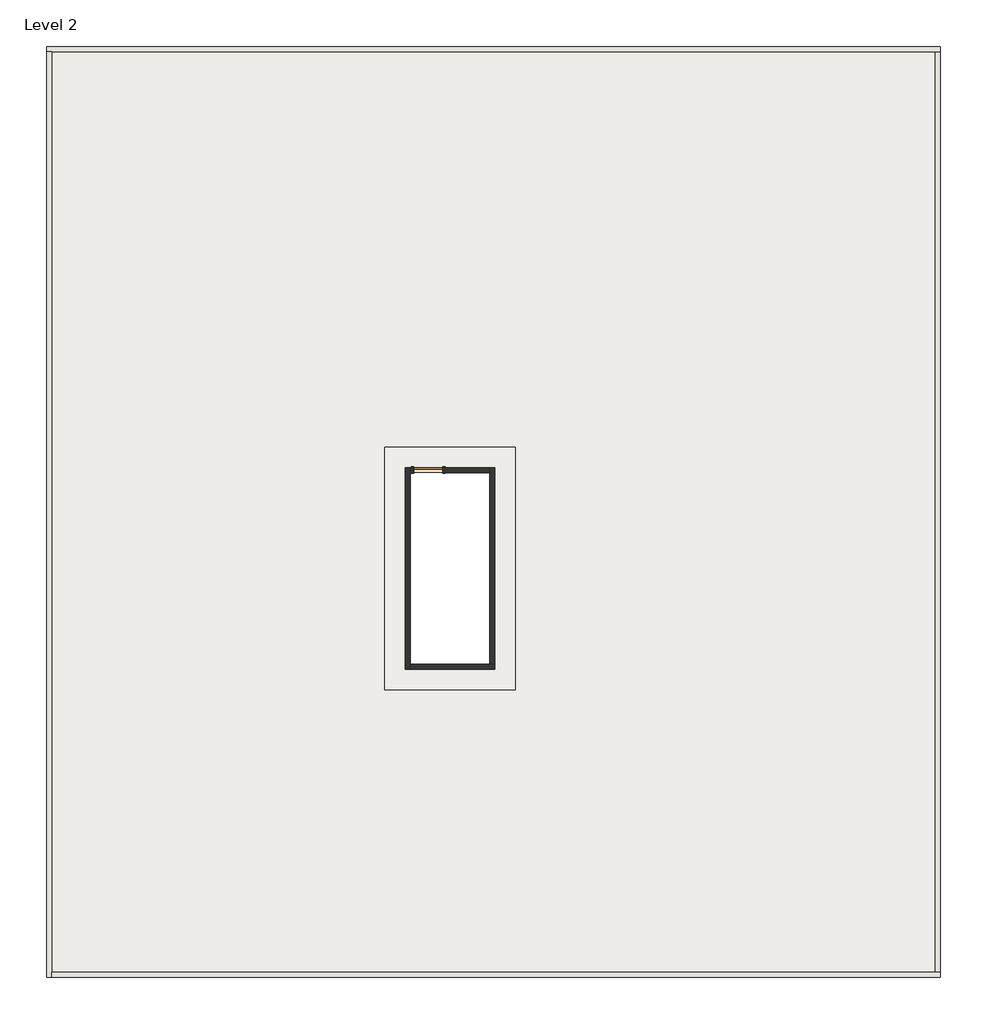
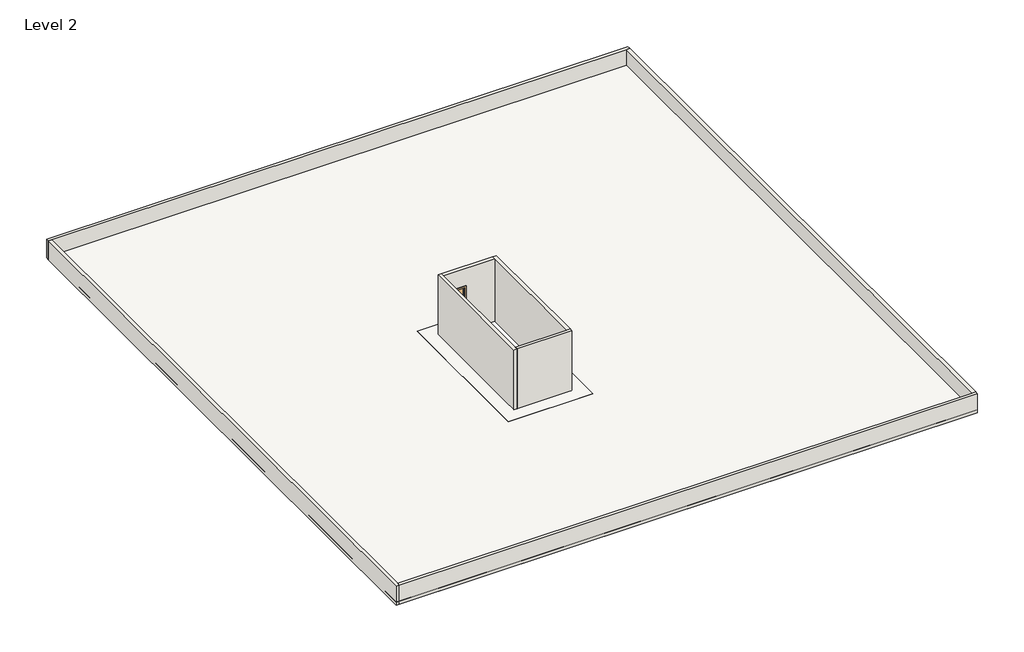
# One storey: 8 walls, 2 roofs, 1 door.
"""IFC4 building model written with IfcOpenShell, lengths in millimetres."""

from ifc_helpers import new_model, si_unit, frame, origin, place, context, project, spatial, polyline, outline, extrude, faceted_brep, transform, mapped, element, save
from components import door_b6e9fca3

model = new_model("IFC4")

# Units and contexts
model_context = context("Model", 3, world=origin())
ifc_project = project(units=[si_unit("LENGTHUNIT", "METRE", prefix="MILLI")], contexts=[model_context])

# Site, building, storey
site = spatial("IfcSite", under=ifc_project)
building = spatial("IfcBuilding", under=site)
storey = spatial("IfcBuildingStorey", under=building, Name="Level 2", Elevation=3048.0)

# Door
placement = place(None, origin())
door_shape = door_b6e9fca3(model_context)
element("IfcDoor", 1, ObjectType="Single-Flush : 34\" x 84\"", at=placement, inside=storey, context=model_context, shape_type="MappedRepresentation", body=[
    mapped(door_shape, transform((-2969.7844485, 1789.3269271, 3048.0), x_axis=(1.0, 0.0, 0.0), y_axis=(0.0, 1.0, 0.0), z_axis=(0.0, 0.0, 1.0))),
])

# Roofs
element("IfcRoof", 2, ObjectType="SLAB", at=placement, inside=storey, context=model_context, shape_type="SweptSolid", body=[
    extrude(outline(polyline([(12308.4014317, 14431.9935985), (12308.4014317, -13355.6064015), (-14366.7474256, -13355.6064015), (-14366.7474256, 14431.9935985), (12308.4014317, 14431.9935985)]), holes=[polyline([(-3503.1844485, 1713.1269271), (-3503.1844485, -4001.8730729), (-1140.9844485, -4001.8730729), (-1140.9844485, 1713.1269271), (-3503.1844485, 1713.1269271)])]), frame((0.0, 0.0, 3048.0), z_axis=(0.0, 0.0, 1.0), x_axis=(1.0, 0.0, 0.0)), (0.0, 0.0, 1.0), 152.4),
])
element("IfcRoof", 3, ObjectType="SLAB", at=placement, inside=storey, context=model_context, shape_type="SweptSolid", body=[
    extrude(outline(polyline([(-378.9844485, -4763.8730729), (-4265.1844485, -4763.8730729), (-4265.1844485, 2475.1269271), (-378.9844485, 2475.1269271), (-378.9844485, -4763.8730729)]), holes=[polyline([(-3503.1844485, 1713.1269271), (-3503.1844485, -4001.8730729), (-1140.9844485, -4001.8730729), (-1140.9844485, 1713.1269271), (-3503.1844485, 1713.1269271)])]), frame((0.0, 0.0, 3048.0), z_axis=(0.0, 0.0, 1.0), x_axis=(1.0, 0.0, 0.0)), (0.0, 0.0, 1.0), 152.4),
])

# Walls
element("IfcWall", 4, ObjectType="6\"", at=placement, inside=storey, context=model_context, shape_type="Brep", body=[
    faceted_brep([(-3655.5844485, 1865.5269271, 3048.0), (-3655.5844485, -4154.2730729, 3048.0), (-3655.5844485, -4154.2730729, 6096.0), (-3655.5844485, 1865.5269271, 6096.0), (-3503.1844485, 1865.5269271, 3048.0), (-3503.1844485, 1865.5269271, 6096.0), (-3503.1844485, 1713.1269271, 6096.0), (-3503.1844485, -4001.8730729, 6096.0), (-3503.1844485, -4154.2730729, 6096.0), (-3503.1844485, -4154.2730729, 3048.0), (-3503.1844485, -4001.8730729, 3048.0), (-3503.1844485, 1713.1269271, 3048.0)], [[[0, 1, 2, 3]], [[4, 5, 6, 7, 8, 9, 10, 11]], [[1, 0, 4, 11, 10, 9]], [[2, 1, 9, 8]], [[0, 3, 5, 4]], [[3, 2, 8, 7, 6, 5]]]),
])
element("IfcWall", 5, ObjectType="6\"", at=placement, inside=storey, context=model_context, shape_type="Brep", body=[
    faceted_brep([(-3503.1844485, -4154.2730729, 3048.0), (-988.5844485, -4154.2730729, 3048.0), (-988.5844485, -4154.2730729, 6096.0), (-3503.1844485, -4154.2730729, 6096.0), (-3503.1844485, -4001.8730729, 3048.0), (-3503.1844485, -4001.8730729, 6096.0), (-1140.9844485, -4001.8730729, 6096.0), (-988.5844485, -4001.8730729, 6096.0), (-988.5844485, -4001.8730729, 3048.0), (-1140.9844485, -4001.8730729, 3048.0)], [[[0, 1, 2, 3]], [[4, 5, 6, 7, 8, 9]], [[1, 0, 4, 9, 8]], [[0, 3, 5, 4]], [[2, 1, 8, 7]], [[3, 2, 7, 6, 5]]]),
])
element("IfcWall", 6, ObjectType="6\"", at=placement, inside=storey, context=model_context, shape_type="Brep", body=[
    faceted_brep([(-988.5844485, -4001.8730729, 3048.0), (-988.5844485, 1865.5269271, 3048.0), (-988.5844485, 1865.5269271, 6096.0), (-988.5844485, -4001.8730729, 6096.0), (-1140.9844485, -4001.8730729, 3048.0), (-1140.9844485, -4001.8730729, 6096.0), (-1140.9844485, 1713.1269271, 6096.0), (-1140.9844485, 1865.5269271, 6096.0), (-1140.9844485, 1865.5269271, 3048.0), (-1140.9844485, 1713.1269271, 3048.0)], [[[0, 1, 2, 3]], [[4, 5, 6, 7, 8, 9]], [[1, 0, 4, 9, 8]], [[0, 3, 5, 4]], [[2, 1, 8, 7]], [[3, 2, 7, 6, 5]]]),
])
element("IfcWall", 7, ObjectType="6\"", at=placement, inside=storey, context=model_context, shape_type="SweptSolid", body=[
    extrude(outline(polyline([(5181.6, -2537.9844485), (3048.0, -2537.9844485), (3048.0, -1140.9844485), (6096.0, -1140.9844485), (6096.0, -3503.1844485), (3048.0, -3503.1844485), (3048.0, -3401.5844485), (5181.6, -3401.5844485), (5181.6, -2537.9844485)])), frame((0.0, 1713.1269271, 0.0), z_axis=(0.0, 1.0, 0.0), x_axis=(0.0, 0.0, 1.0)), (0.0, 0.0, 1.0), 152.4),
])
element("IfcWall", 8, ObjectType="6\" 2", at=placement, inside=storey, context=model_context, shape_type="Brep", body=[
    faceted_brep([(12308.4014317, 14431.9935985, 3048.0), (-14366.7474256, 14431.9935985, 3048.0), (-14366.7474256, 14431.9935985, 3962.4), (12308.4014317, 14431.9935985, 3962.4), (12308.4014317, 14279.5935985, 3048.0), (12308.4014317, 14279.5935985, 3962.4), (12156.0014317, 14279.5935985, 3962.4), (-14214.3474256, 14279.5935985, 3962.4), (-14366.7474256, 14279.5935985, 3962.4), (-14366.7474256, 14279.5935985, 3048.0), (-14214.3474256, 14279.5935985, 3048.0), (12156.0014317, 14279.5935985, 3048.0)], [[[0, 1, 2, 3]], [[4, 5, 6, 7, 8, 9, 10, 11]], [[1, 0, 4, 11, 10, 9]], [[3, 2, 8, 7, 6, 5]], [[2, 1, 9, 8]], [[0, 3, 5, 4]]]),
])
element("IfcWall", 9, ObjectType="6\" 2", at=placement, inside=storey, context=model_context, shape_type="Brep", body=[
    faceted_brep([(-14366.7474256, 14279.5935985, 3048.0), (-14366.7474256, -13355.6064015, 3048.0), (-14366.7474256, -13355.6064015, 3962.4), (-14366.7474256, 14279.5935985, 3962.4), (-14214.3474256, 14279.5935985, 3048.0), (-14214.3474256, 14279.5935985, 3962.4), (-14214.3474256, -13203.2064015, 3962.4), (-14214.3474256, -13355.6064015, 3962.4), (-14214.3474256, -13355.6064015, 3048.0), (-14214.3474256, -13203.2064015, 3048.0)], [[[0, 1, 2, 3]], [[4, 5, 6, 7, 8, 9]], [[1, 0, 4, 9, 8]], [[3, 2, 7, 6, 5]], [[0, 3, 5, 4]], [[2, 1, 8, 7]]]),
])
element("IfcWall", 10, ObjectType="6\" 2", at=placement, inside=storey, context=model_context, shape_type="Brep", body=[
    faceted_brep([(-14214.3474256, -13355.6064015, 3048.0), (12308.4014317, -13355.6064015, 3048.0), (12308.4014317, -13355.6064015, 3962.4), (-14214.3474256, -13355.6064015, 3962.4), (-14214.3474256, -13203.2064015, 3048.0), (-14214.3474256, -13203.2064015, 3962.4), (12156.0014317, -13203.2064015, 3962.4), (12308.4014317, -13203.2064015, 3962.4), (12308.4014317, -13203.2064015, 3048.0), (12156.0014317, -13203.2064015, 3048.0)], [[[0, 1, 2, 3]], [[4, 5, 6, 7, 8, 9]], [[1, 0, 4, 9, 8]], [[3, 2, 7, 6, 5]], [[0, 3, 5, 4]], [[2, 1, 8, 7]]]),
])
element("IfcWall", 11, ObjectType="6\" 2", at=placement, inside=storey, context=model_context, shape_type="SweptSolid", body=[
    extrude(outline(polyline([(12308.4014317, 14279.5935985), (12308.4014317, -13203.2064015), (12156.0014317, -13203.2064015), (12156.0014317, 14279.5935985), (12308.4014317, 14279.5935985)])), frame((0.0, 0.0, 3048.0), z_axis=(0.0, 0.0, 1.0), x_axis=(1.0, 0.0, 0.0)), (0.0, 0.0, 1.0), 914.4),
])

save(model, "model.ifc")

# Revit data of these elements
# Type "Single-Flush : 34\" x 84\""
#   Type Mark = "2"
#   Construction Type Id = "MDOOR"
#   Assembly Code = "C1020"
#   Analytic Construction = "Metal"
#   Thickness = 0' - 2"
#   Heat Transfer Coefficient (U) = 0.651978 BTU/(h·ft²·°F)
#   Height = 7' - 0"
#   Trim Projection Ext = 0' - 1"
#   Trim Projection Int = 0' - 1"
#   Trim Width = 0' - 3"
#   Width = 2' - 10"
#   Define Thermal Properties by = 1
#   Define Thermal Properties by = 1
#   Door Material = Door - Panel
#   Frame Material = Door - Frame
#   Visual Light Transmittance = 0
#   Solar Heat Gain Coefficient = 0
#   Function = (empty or 0)
#   Wall Closure = (empty or 0)
# Type "SLAB"
#   Assembly Code = "B1020"
#   Layers, outside or top first: 0' - 6" "SLAB" (function 1)
# Type "6\""
#   Assembly Code = "B2010"
#   Layers, outside or top first: 0' - 6" "6\" WALL" (function 1)
# Type "6\" 2"
#   Assembly Code = "B2010"
#   Layers, outside or top first: 0' - 6" "6\" WALL" (function 1)
# Element 1 (IfcDoor, "Single-Flush : 34\" x 84\"")
#   Phase Created = New Construction
#   Materials on its faces: "Door - Frame", "Door - Panel"
# Elements 2, 3 (IfcRoof, "SLAB")
#   built-in parameter 1001705 = 10.5 (stored number, unit not read)
#   built-in parameter 1001710 = 33615
#   Phase Created = New Construction
#   Materials on its faces: "SLAB"
# Elements 4, 5, 6, 7 (IfcWall, "6\"")
#   Top Offset = 0' - 0"
#   Base Offset = 0' - 0"
#   Unconnected Height = 10' - 0"
#   wall height = 10' - 0"
#   Phase Created = New Construction
#   Base Constraint = Level 2
#   Materials on its faces: "6\" WALL"
# Elements 8, 9, 10, 11 (IfcWall, "6\" 2")
#   Top Offset = 0' - 0"
#   Base Offset = 0' - 0"
#   Unconnected Height = 3' - 0"
#   wall height = 3' - 0"
#   Phase Created = New Construction
#   Base Constraint = Level 2
#   Materials on its faces: "6\" WALL"
# Materials
#   "Door - Panel": class "Wood", colour RGB 210 159 95, transparency 0, Cost = 0
#   "Door - Frame": colour RGB 118 70 51, transparency 0, Cost = 0
#   "SLAB": class "Generic", colour RGB 120 120 120, transparency 0, Cost = 0
#   "6\" WALL": class "Generic", colour RGB 120 120 120, transparency 0, Cost = 0
